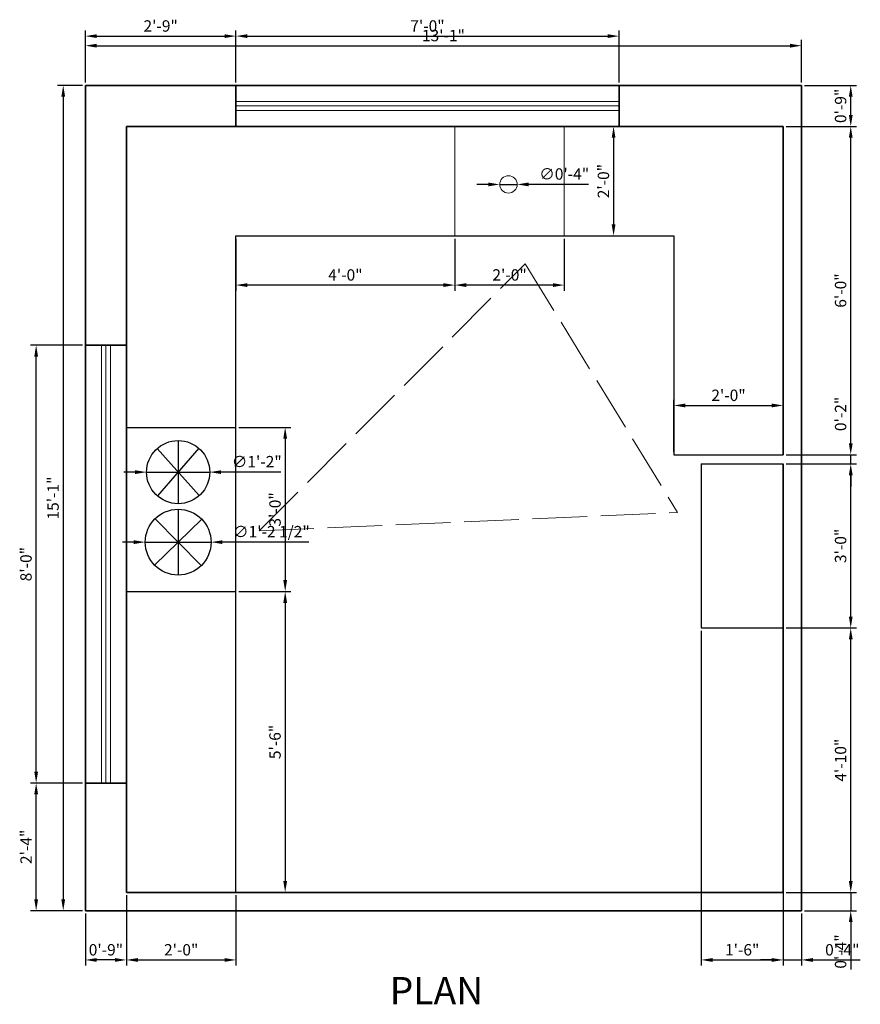
# Model space of a CAD drawing. Units: inches. Extents: x 125 to 951, y 142 to 358.
# Tile 1 of 4: x 125 to 309, y 142 to 358. Entities that reach past the tile are written whole.
import ezdxf

# ---------------------------------------------------------------- set-up
doc = ezdxf.new("R2010")
doc.units = ezdxf.units.IN
doc.linetypes.add('ACAD_ISO02W100', pattern=[15, 12, -3])
for name, color, linetype, lineweight in [('A-ANNO-DIMS', 2, 'Continuous', 18), ('A-ANNO-TEXT', 7, 'Continuous', 25), ('A-ANNO-WORK', 3, 'ACAD_ISO02W100', 13), ('A-EQPM', 8, 'Continuous', 25), ('A-FLOR-CNTR', 30, 'Continuous', 25), ('A-FLOR-FIXT', 9, 'Continuous', 18), ('A-GLAZ', 4, 'Continuous', 18), ('A-WALL', 7, 'Continuous', 35)]:
    doc.layers.add(name, color=color, linetype=linetype, lineweight=lineweight)
doc.styles.get("Standard").update_dxf_attribs({"font": 'arial.ttf'})
doc.dimstyles.new('ISO-25', dxfattribs={"dimtxt": 2.5, "dimasz": 2.5, "dimexe": 1.25, "dimexo": 0.625, "dimtad": 1, "dimlunit": 3, "dimtxsty": 'Standard', "dimcen": 2.5, "dimadec": 0, "dimazin": 0, "dimtfac": 1, "dimtmove": 0, "dimatfit": 3, "dimfxl": 1, "dimarcsym": 0})

# ---------------------------------------------------------------- blocks, each defined once
blk = doc.blocks.new('*D1')
at = {"layer": 'A-ANNO-DIMS', "color": 0, "lineweight": -2, "transparency": 16777216}
for p, q in [((138.96, 344.03), (138.96, 353.36)), ((141.46, 352.11), (293.46, 352.11)), ((295.96, 344.03), (295.96, 353.36))]:
    blk.add_line(p, q, dxfattribs=at)
at = {"layer": 'A-ANNO-DIMS', "color": 0, "transparency": 16777216}
for points in [[(141.46, 352.53), (141.46, 351.69), (138.96, 352.11)], [(293.46, 352.53), (293.46, 351.69), (295.96, 352.11)]]:
    blk.add_solid(points, dxfattribs=at)
at = {"layer": 'Defpoints', "color": 0, "transparency": 16777216}
for p in [(295.96, 352.11), (138.96, 343.41), (295.96, 343.41)]:
    blk.add_point(p, dxfattribs=at)
at = {"layer": 'A-ANNO-DIMS', "color": 0, "transparency": 16777216, "insert": (217.46, 354.01), "char_height": 2.5, "attachment_point": 5}
blk.add_mtext('13\'-1"', dxfattribs=at)
blk = doc.blocks.new('*D2')
at = {"layer": 'A-ANNO-DIMS', "color": 0, "lineweight": -2, "transparency": 16777216}
for p, q in [((138.34, 343.41), (132.85, 343.41)), ((134.1, 340.91), (134.1, 164.91)), ((138.34, 162.41), (132.85, 162.41))]:
    blk.add_line(p, q, dxfattribs=at)
at = {"layer": 'A-ANNO-DIMS', "color": 0, "transparency": 16777216}
for points in [[(133.68, 340.91), (134.51, 340.91), (134.1, 343.41)], [(133.68, 164.91), (134.51, 164.91), (134.1, 162.41)]]:
    blk.add_solid(points, dxfattribs=at)
at = {"layer": 'Defpoints', "color": 0, "transparency": 16777216}
for p in [(138.96, 343.41), (134.1, 162.41), (138.96, 162.41)]:
    blk.add_point(p, dxfattribs=at)
at = {"layer": 'A-ANNO-DIMS', "color": 0, "transparency": 16777216, "insert": (132.19, 252.91), "char_height": 2.5, "attachment_point": 5, "rotation": 90}
blk.add_mtext('15\'-1"', dxfattribs=at)
blk = doc.blocks.new('*D21')
at = {"layer": 'A-ANNO-DIMS', "color": 0, "lineweight": -2, "transparency": 16777216}
for p, q in [((138.96, 344.03), (138.96, 355.46)), ((141.46, 354.21), (169.46, 354.21)), ((171.96, 344.03), (171.96, 355.46))]:
    blk.add_line(p, q, dxfattribs=at)
at = {"layer": 'A-ANNO-DIMS', "color": 0, "transparency": 16777216}
for points in [[(141.46, 354.62), (141.46, 353.79), (138.96, 354.21)], [(169.46, 354.62), (169.46, 353.79), (171.96, 354.21)]]:
    blk.add_solid(points, dxfattribs=at)
at = {"layer": 'Defpoints', "color": 0, "transparency": 16777216}
for p in [(171.96, 354.21), (138.96, 343.41), (171.96, 343.41)]:
    blk.add_point(p, dxfattribs=at)
at = {"layer": 'A-ANNO-DIMS', "color": 0, "transparency": 16777216, "insert": (155.46, 356.11), "char_height": 2.5, "attachment_point": 5}
blk.add_mtext('2\'-9"', dxfattribs=at)
blk = doc.blocks.new('*D22')
at = {"layer": 'A-ANNO-DIMS', "color": 0, "lineweight": -2, "transparency": 16777216}
for p, q in [((171.96, 344.03), (171.96, 355.46)), ((174.46, 354.21), (253.46, 354.21)), ((255.96, 344.03), (255.96, 355.46))]:
    blk.add_line(p, q, dxfattribs=at)
at = {"layer": 'A-ANNO-DIMS', "color": 0, "transparency": 16777216}
for points in [[(174.46, 354.62), (174.46, 353.79), (171.96, 354.21)], [(253.46, 354.62), (253.46, 353.79), (255.96, 354.21)]]:
    blk.add_solid(points, dxfattribs=at)
at = {"layer": 'Defpoints', "color": 0, "transparency": 16777216}
for p in [(255.96, 354.21), (171.96, 343.41), (255.96, 343.41)]:
    blk.add_point(p, dxfattribs=at)
at = {"layer": 'A-ANNO-DIMS', "color": 0, "transparency": 16777216, "insert": (213.96, 356.11), "char_height": 2.5, "attachment_point": 5}
blk.add_mtext('7\'-0"', dxfattribs=at)
blk = doc.blocks.new('*D23')
at = {"layer": 'A-ANNO-DIMS', "color": 0, "lineweight": -2, "transparency": 16777216}
for p, q in [((138.34, 286.41), (126.91, 286.41)), ((128.16, 192.91), (128.16, 283.91)), ((138.34, 190.41), (126.91, 190.41))]:
    blk.add_line(p, q, dxfattribs=at)
at = {"layer": 'A-ANNO-DIMS', "color": 0, "transparency": 16777216}
for points in [[(127.75, 283.91), (128.58, 283.91), (128.16, 286.41)], [(127.75, 192.91), (128.58, 192.91), (128.16, 190.41)]]:
    blk.add_solid(points, dxfattribs=at)
at = {"layer": 'Defpoints', "color": 0, "transparency": 16777216}
for p in [(128.16, 286.41), (138.96, 286.41), (138.96, 190.41)]:
    blk.add_point(p, dxfattribs=at)
at = {"layer": 'A-ANNO-DIMS', "color": 0, "transparency": 16777216, "insert": (126.26, 238.41), "char_height": 2.5, "attachment_point": 5, "rotation": 90}
blk.add_mtext('8\'-0"', dxfattribs=at)
blk = doc.blocks.new('*D24')
at = {"layer": 'A-ANNO-DIMS', "color": 0, "lineweight": -2, "transparency": 16777216}
for p, q in [((138.34, 190.41), (126.91, 190.41)), ((128.16, 164.91), (128.16, 187.91)), ((138.34, 162.41), (126.91, 162.41))]:
    blk.add_line(p, q, dxfattribs=at)
at = {"layer": 'A-ANNO-DIMS', "color": 0, "transparency": 16777216}
for points in [[(127.75, 187.91), (128.58, 187.91), (128.16, 190.41)], [(127.75, 164.91), (128.58, 164.91), (128.16, 162.41)]]:
    blk.add_solid(points, dxfattribs=at)
at = {"layer": 'Defpoints', "color": 0, "transparency": 16777216}
for p in [(128.16, 190.41), (138.96, 190.41), (138.96, 162.41)]:
    blk.add_point(p, dxfattribs=at)
at = {"layer": 'A-ANNO-DIMS', "color": 0, "transparency": 16777216, "insert": (126.28, 176.41), "char_height": 2.5, "attachment_point": 5, "rotation": 90}
blk.add_mtext('2\'-4"', dxfattribs=at)
blk = doc.blocks.new('*D25')
at = {"layer": 'A-ANNO-DIMS', "color": 0, "lineweight": -2, "transparency": 16777216}
for p, q in [((147.96, 165.78), (147.96, 150.36)), ((171.96, 165.78), (171.96, 150.36)), ((150.46, 151.61), (169.46, 151.61))]:
    blk.add_line(p, q, dxfattribs=at)
at = {"layer": 'A-ANNO-DIMS', "color": 0, "transparency": 16777216}
for points in [[(150.46, 152.02), (150.46, 151.19), (147.96, 151.61)], [(169.46, 152.02), (169.46, 151.19), (171.96, 151.61)]]:
    blk.add_solid(points, dxfattribs=at)
at = {"layer": 'Defpoints', "color": 0, "transparency": 16777216}
for p in [(147.96, 166.41), (171.96, 166.41), (171.96, 151.61)]:
    blk.add_point(p, dxfattribs=at)
at = {"layer": 'A-ANNO-DIMS', "color": 0, "transparency": 16777216, "insert": (159.96, 153.51), "char_height": 2.5, "attachment_point": 5}
blk.add_mtext('2\'-0"', dxfattribs=at)
blk = doc.blocks.new('*D26')
at = {"layer": 'A-ANNO-DIMS', "color": 0, "lineweight": -2, "transparency": 16777216}
for p, q in [((171.96, 309.78), (171.96, 298.36)), ((219.96, 309.78), (219.96, 298.36)), ((217.46, 299.61), (174.46, 299.61))]:
    blk.add_line(p, q, dxfattribs=at)
at = {"layer": 'A-ANNO-DIMS', "color": 0, "transparency": 16777216}
for points in [[(174.46, 300.02), (174.46, 299.19), (171.96, 299.61)], [(217.46, 300.02), (217.46, 299.19), (219.96, 299.61)]]:
    blk.add_solid(points, dxfattribs=at)
at = {"layer": 'Defpoints', "color": 0, "transparency": 16777216}
for p in [(171.96, 310.41), (219.96, 310.41), (171.96, 299.61)]:
    blk.add_point(p, dxfattribs=at)
at = {"layer": 'A-ANNO-DIMS', "color": 0, "transparency": 16777216, "insert": (195.96, 301.51), "char_height": 2.5, "attachment_point": 5}
blk.add_mtext('4\'-0"', dxfattribs=at)
blk = doc.blocks.new('*D27')
at = {"layer": 'A-ANNO-DIMS', "color": 0, "lineweight": -2, "transparency": 16777216}
for p, q in [((219.96, 309.78), (219.96, 298.36)), ((243.96, 309.78), (243.96, 298.36)), ((241.46, 299.61), (222.46, 299.61))]:
    blk.add_line(p, q, dxfattribs=at)
at = {"layer": 'A-ANNO-DIMS', "color": 0, "transparency": 16777216}
for points in [[(222.46, 300.02), (222.46, 299.19), (219.96, 299.61)], [(241.46, 300.02), (241.46, 299.19), (243.96, 299.61)]]:
    blk.add_solid(points, dxfattribs=at)
at = {"layer": 'Defpoints', "color": 0, "transparency": 16777216}
for p in [(219.96, 310.41), (243.96, 310.41), (219.96, 299.61)]:
    blk.add_point(p, dxfattribs=at)
at = {"layer": 'A-ANNO-DIMS', "color": 0, "transparency": 16777216, "insert": (231.96, 301.51), "char_height": 2.5, "attachment_point": 5}
blk.add_mtext('2\'-0"', dxfattribs=at)
blk = doc.blocks.new('*D28')
at = {"layer": 'A-ANNO-DIMS', "color": 0, "lineweight": -2, "transparency": 16777216}
for p, q in [((172.59, 232.41), (184.01, 232.41)), ((182.76, 229.91), (182.76, 168.91)), ((172.59, 166.41), (184.01, 166.41))]:
    blk.add_line(p, q, dxfattribs=at)
at = {"layer": 'A-ANNO-DIMS', "color": 0, "transparency": 16777216}
for points in [[(182.35, 229.91), (183.18, 229.91), (182.76, 232.41)], [(182.35, 168.91), (183.18, 168.91), (182.76, 166.41)]]:
    blk.add_solid(points, dxfattribs=at)
at = {"layer": 'Defpoints', "color": 0, "transparency": 16777216}
for p in [(171.96, 232.41), (171.96, 166.41), (182.76, 166.41)]:
    blk.add_point(p, dxfattribs=at)
at = {"layer": 'A-ANNO-DIMS', "color": 0, "transparency": 16777216, "insert": (180.86, 199.41), "char_height": 2.5, "attachment_point": 5, "rotation": 90}
blk.add_mtext('5\'-6"', dxfattribs=at)
blk = doc.blocks.new('*D29')
at = {"layer": 'A-ANNO-DIMS', "color": 0, "lineweight": -2, "transparency": 16777216}
for p, q in [((172.59, 268.41), (184.01, 268.41)), ((182.76, 265.91), (182.76, 234.91)), ((172.59, 232.41), (184.01, 232.41))]:
    blk.add_line(p, q, dxfattribs=at)
at = {"layer": 'A-ANNO-DIMS', "color": 0, "transparency": 16777216}
for points in [[(182.35, 265.91), (183.18, 265.91), (182.76, 268.41)], [(182.35, 234.91), (183.18, 234.91), (182.76, 232.41)]]:
    blk.add_solid(points, dxfattribs=at)
at = {"layer": 'Defpoints', "color": 0, "transparency": 16777216}
for p in [(171.96, 268.41), (171.96, 232.41), (182.76, 232.41)]:
    blk.add_point(p, dxfattribs=at)
at = {"layer": 'A-ANNO-DIMS', "color": 0, "transparency": 16777216, "insert": (180.86, 250.41), "char_height": 2.5, "attachment_point": 5, "rotation": 90}
blk.add_mtext('3\'-0"', dxfattribs=at)
blk = doc.blocks.new('*D30')
at = {"layer": 'A-ANNO-DIMS', "color": 0, "lineweight": -2, "transparency": 16777216}
for p, q in [((292.59, 334.41), (308.01, 334.41)), ((306.76, 264.91), (306.76, 331.91)), ((292.59, 262.41), (308.01, 262.41))]:
    blk.add_line(p, q, dxfattribs=at)
at = {"layer": 'A-ANNO-DIMS', "color": 0, "transparency": 16777216}
for points in [[(306.35, 331.91), (307.18, 331.91), (306.76, 334.41)], [(306.35, 264.91), (307.18, 264.91), (306.76, 262.41)]]:
    blk.add_solid(points, dxfattribs=at)
at = {"layer": 'Defpoints', "color": 0, "transparency": 16777216}
for p in [(291.96, 334.41), (306.76, 334.41), (291.96, 262.41)]:
    blk.add_point(p, dxfattribs=at)
at = {"layer": 'A-ANNO-DIMS', "color": 0, "transparency": 16777216, "insert": (304.86, 298.41), "char_height": 2.5, "attachment_point": 5, "rotation": 90}
blk.add_mtext('6\'-0"', dxfattribs=at)
blk = doc.blocks.new('*D31')
at = {"layer": 'A-ANNO-DIMS', "color": 0, "lineweight": -2, "transparency": 16777216}
for p, q in [((273.96, 223.78), (273.96, 150.36)), ((291.96, 223.78), (291.96, 150.36)), ((276.46, 151.61), (289.46, 151.61))]:
    blk.add_line(p, q, dxfattribs=at)
at = {"layer": 'A-ANNO-DIMS', "color": 0, "transparency": 16777216}
for points in [[(276.46, 152.02), (276.46, 151.19), (273.96, 151.61)], [(289.46, 152.02), (289.46, 151.19), (291.96, 151.61)]]:
    blk.add_solid(points, dxfattribs=at)
at = {"layer": 'Defpoints', "color": 0, "transparency": 16777216}
for p in [(273.96, 224.41), (291.96, 224.41), (291.96, 151.61)]:
    blk.add_point(p, dxfattribs=at)
at = {"layer": 'A-ANNO-DIMS', "color": 0, "transparency": 16777216, "insert": (282.96, 153.51), "char_height": 2.5, "attachment_point": 5}
blk.add_mtext('1\'-6"', dxfattribs=at)
blk = doc.blocks.new('*D32')
at = {"layer": 'A-ANNO-DIMS', "color": 0, "lineweight": -2, "transparency": 16777216}
for p, q in [((292.59, 260.41), (308.01, 260.41)), ((306.76, 226.91), (306.76, 257.91)), ((292.59, 224.41), (308.01, 224.41))]:
    blk.add_line(p, q, dxfattribs=at)
at = {"layer": 'A-ANNO-DIMS', "color": 0, "transparency": 16777216}
for points in [[(306.35, 257.91), (307.18, 257.91), (306.76, 260.41)], [(306.35, 226.91), (307.18, 226.91), (306.76, 224.41)]]:
    blk.add_solid(points, dxfattribs=at)
at = {"layer": 'Defpoints', "color": 0, "transparency": 16777216}
for p in [(291.96, 260.41), (306.76, 260.41), (291.96, 224.41)]:
    blk.add_point(p, dxfattribs=at)
at = {"layer": 'A-ANNO-DIMS', "color": 0, "transparency": 16777216, "insert": (304.86, 242.41), "char_height": 2.5, "attachment_point": 5, "rotation": 90}
blk.add_mtext('3\'-0"', dxfattribs=at)
blk = doc.blocks.new('*D33')
at = {"layer": 'A-ANNO-DIMS', "color": 0, "lineweight": -2, "transparency": 16777216}
for p, q in [((292.59, 224.41), (308.01, 224.41)), ((306.76, 168.91), (306.76, 221.91)), ((292.59, 166.41), (308.01, 166.41))]:
    blk.add_line(p, q, dxfattribs=at)
at = {"layer": 'A-ANNO-DIMS', "color": 0, "transparency": 16777216}
for points in [[(306.35, 221.91), (307.18, 221.91), (306.76, 224.41)], [(306.35, 168.91), (307.18, 168.91), (306.76, 166.41)]]:
    blk.add_solid(points, dxfattribs=at)
at = {"layer": 'Defpoints', "color": 0, "transparency": 16777216}
for p in [(291.96, 224.41), (306.76, 224.41), (291.96, 166.41)]:
    blk.add_point(p, dxfattribs=at)
at = {"layer": 'A-ANNO-DIMS', "color": 0, "transparency": 16777216, "insert": (304.86, 195.41), "char_height": 2.5, "attachment_point": 5, "rotation": 90}
blk.add_mtext('4\'-10"', dxfattribs=at)
blk = doc.blocks.new('*D34')
at = {"layer": 'A-ANNO-DIMS', "color": 0, "lineweight": -2, "transparency": 16777216}
for p, q in [((147.96, 165.78), (147.96, 150.36)), ((138.96, 161.78), (138.96, 150.36)), ((145.46, 151.61), (141.46, 151.61))]:
    blk.add_line(p, q, dxfattribs=at)
at = {"layer": 'A-ANNO-DIMS', "color": 0, "transparency": 16777216}
for points in [[(141.46, 152.02), (141.46, 151.19), (138.96, 151.61)], [(145.46, 152.02), (145.46, 151.19), (147.96, 151.61)]]:
    blk.add_solid(points, dxfattribs=at)
at = {"layer": 'Defpoints', "color": 0, "transparency": 16777216}
for p in [(147.96, 166.41), (138.96, 162.41), (138.96, 151.61)]:
    blk.add_point(p, dxfattribs=at)
at = {"layer": 'A-ANNO-DIMS', "color": 0, "transparency": 16777216, "insert": (143.46, 153.51), "char_height": 2.5, "attachment_point": 5}
blk.add_mtext('0\'-9"', dxfattribs=at)
blk = doc.blocks.new('*D35')
at = {"layer": 'A-ANNO-DIMS', "color": 0, "lineweight": -2, "transparency": 16777216}
for p, q in [((291.96, 165.78), (291.96, 150.36)), ((295.96, 161.78), (295.96, 150.36)), ((289.46, 151.61), (286.96, 151.61)), ((291.96, 151.61), (295.96, 151.61)), ((298.46, 151.61), (308.86, 151.61))]:
    blk.add_line(p, q, dxfattribs=at)
at = {"layer": 'A-ANNO-DIMS', "color": 0, "transparency": 16777216}
for points in [[(289.46, 152.02), (289.46, 151.19), (291.96, 151.61)], [(298.46, 152.02), (298.46, 151.19), (295.96, 151.61)]]:
    blk.add_solid(points, dxfattribs=at)
at = {"layer": 'Defpoints', "color": 0, "transparency": 16777216}
for p in [(291.96, 166.41), (295.96, 162.41), (295.96, 151.61)]:
    blk.add_point(p, dxfattribs=at)
at = {"layer": 'A-ANNO-DIMS', "color": 0, "transparency": 16777216, "insert": (304.91, 153.51), "char_height": 2.5, "attachment_point": 5}
blk.add_mtext('0\'-4"', dxfattribs=at)
blk = doc.blocks.new('*D36')
at = {"layer": 'A-ANNO-DIMS', "color": 0, "lineweight": -2, "transparency": 16777216}
for p, q in [((296.59, 343.41), (308.01, 343.41)), ((306.76, 336.91), (306.76, 340.91)), ((292.59, 334.41), (308.01, 334.41))]:
    blk.add_line(p, q, dxfattribs=at)
at = {"layer": 'A-ANNO-DIMS', "color": 0, "transparency": 16777216}
for points in [[(306.35, 340.91), (307.18, 340.91), (306.76, 343.41)], [(306.35, 336.91), (307.18, 336.91), (306.76, 334.41)]]:
    blk.add_solid(points, dxfattribs=at)
at = {"layer": 'Defpoints', "color": 0, "transparency": 16777216}
for p in [(295.96, 343.41), (306.76, 343.41), (291.96, 334.41)]:
    blk.add_point(p, dxfattribs=at)
at = {"layer": 'A-ANNO-DIMS', "color": 0, "transparency": 16777216, "insert": (304.86, 338.91), "char_height": 2.5, "attachment_point": 5, "rotation": 90}
blk.add_mtext('0\'-9"', dxfattribs=at)
blk = doc.blocks.new('*D37')
at = {"layer": 'A-ANNO-DIMS', "color": 0, "lineweight": -2, "transparency": 16777216}
for p, q in [((306.76, 168.91), (306.76, 171.41)), ((292.59, 166.41), (308.01, 166.41)), ((306.76, 166.41), (306.76, 162.41)), ((296.59, 162.41), (308.01, 162.41)), ((306.76, 159.91), (306.76, 149.51))]:
    blk.add_line(p, q, dxfattribs=at)
at = {"layer": 'A-ANNO-DIMS', "color": 0, "transparency": 16777216}
for points in [[(306.35, 168.91), (307.18, 168.91), (306.76, 166.41)], [(306.35, 159.91), (307.18, 159.91), (306.76, 162.41)]]:
    blk.add_solid(points, dxfattribs=at)
at = {"layer": 'Defpoints', "color": 0, "transparency": 16777216}
for p in [(291.96, 166.41), (295.96, 162.41), (306.76, 162.41)]:
    blk.add_point(p, dxfattribs=at)
at = {"layer": 'A-ANNO-DIMS', "color": 0, "transparency": 16777216, "insert": (304.86, 153.46), "char_height": 2.5, "attachment_point": 5, "rotation": 90}
blk.add_mtext('0\'-4"', dxfattribs=at)
blk = doc.blocks.new('*D38')
at = {"layer": 'A-ANNO-DIMS', "color": 0, "lineweight": -2, "transparency": 16777216}
for p, q in [((244.59, 334.41), (256.01, 334.41)), ((254.76, 331.91), (254.76, 312.91)), ((244.59, 310.41), (256.01, 310.41))]:
    blk.add_line(p, q, dxfattribs=at)
at = {"layer": 'A-ANNO-DIMS', "color": 0, "transparency": 16777216}
for points in [[(254.35, 331.91), (255.18, 331.91), (254.76, 334.41)], [(254.35, 312.91), (255.18, 312.91), (254.76, 310.41)]]:
    blk.add_solid(points, dxfattribs=at)
at = {"layer": 'Defpoints', "color": 0, "transparency": 16777216}
for p in [(243.96, 334.41), (243.96, 310.41), (254.76, 310.41)]:
    blk.add_point(p, dxfattribs=at)
at = {"layer": 'A-ANNO-DIMS', "color": 0, "transparency": 16777216, "insert": (252.86, 322.41), "char_height": 2.5, "attachment_point": 5, "rotation": 90}
blk.add_mtext('2\'-0"', dxfattribs=at)
blk = doc.blocks.new('*D39')
at = {"layer": 'A-ANNO-DIMS', "color": 0, "lineweight": -2, "transparency": 16777216}
for p, q in [((267.96, 263.03), (267.96, 274.46)), ((291.96, 263.03), (291.96, 274.46)), ((270.46, 273.21), (289.46, 273.21))]:
    blk.add_line(p, q, dxfattribs=at)
at = {"layer": 'A-ANNO-DIMS', "color": 0, "transparency": 16777216}
for points in [[(270.46, 273.62), (270.46, 272.79), (267.96, 273.21)], [(289.46, 273.62), (289.46, 272.79), (291.96, 273.21)]]:
    blk.add_solid(points, dxfattribs=at)
at = {"layer": 'Defpoints', "color": 0, "transparency": 16777216}
for p in [(291.96, 273.21), (267.96, 262.41), (291.96, 262.41)]:
    blk.add_point(p, dxfattribs=at)
at = {"layer": 'A-ANNO-DIMS', "color": 0, "transparency": 16777216, "insert": (279.96, 275.11), "char_height": 2.5, "attachment_point": 5}
blk.add_mtext('2\'-0"', dxfattribs=at)
blk = doc.blocks.new('*D40')
at = {"layer": 'A-ANNO-DIMS', "color": 0, "lineweight": -2, "transparency": 16777216}
for p, q in [((306.76, 264.91), (306.76, 275.3)), ((292.59, 262.41), (308.01, 262.41)), ((306.76, 260.41), (306.76, 262.41)), ((292.59, 260.41), (308.01, 260.41)), ((306.76, 257.91), (306.76, 255.41))]:
    blk.add_line(p, q, dxfattribs=at)
at = {"layer": 'A-ANNO-DIMS', "color": 0, "transparency": 16777216}
for points in [[(306.35, 264.91), (307.18, 264.91), (306.76, 262.41)], [(306.35, 257.91), (307.18, 257.91), (306.76, 260.41)]]:
    blk.add_solid(points, dxfattribs=at)
at = {"layer": 'Defpoints', "color": 0, "transparency": 16777216}
for p in [(291.96, 262.41), (306.76, 262.41), (291.96, 260.41)]:
    blk.add_point(p, dxfattribs=at)
at = {"layer": 'A-ANNO-DIMS', "color": 0, "transparency": 16777216, "insert": (304.86, 271.35), "char_height": 2.5, "attachment_point": 5, "rotation": 90}
blk.add_mtext('0\'-2"', dxfattribs=at)
blk = doc.blocks.new('*D72')
at = {"layer": 'A-ANNO-DIMS', "color": 0, "lineweight": -2, "transparency": 16777216}
for p, q in [((149.57, 243.23), (147.07, 243.23)), ((152.07, 243.23), (166.52, 243.23)), ((187.96, 243.23), (169.02, 243.23))]:
    blk.add_line(p, q, dxfattribs=at)
at = {"layer": 'A-ANNO-DIMS', "color": 0, "transparency": 16777216}
for points in [[(149.57, 243.65), (149.57, 242.82), (152.07, 243.23)], [(169.02, 243.65), (169.02, 242.82), (166.52, 243.23)]]:
    blk.add_solid(points, dxfattribs=at)
at = {"layer": 'Defpoints', "color": 0, "transparency": 16777216}
for p in [(152.07, 243.23), (166.52, 243.23)]:
    blk.add_point(p, dxfattribs=at)
at = {"layer": 'A-ANNO-DIMS', "color": 0, "transparency": 16777216, "insert": (179.74, 245.21), "char_height": 2.5, "attachment_point": 5, "rotation": 0.0037}
blk.add_mtext('∅1\'-2 1/2"', dxfattribs=at)
blk = doc.blocks.new('*D73')
at = {"layer": 'A-ANNO-DIMS', "color": 0, "lineweight": -2, "transparency": 16777216}
for p, q in [((149.87, 258.59), (147.37, 258.59)), ((152.37, 258.59), (166.22, 258.59)), ((181.84, 258.59), (168.72, 258.59))]:
    blk.add_line(p, q, dxfattribs=at)
at = {"layer": 'A-ANNO-DIMS', "color": 0, "transparency": 16777216}
for points in [[(149.87, 259), (149.87, 258.17), (152.37, 258.59)], [(168.72, 259), (168.72, 258.17), (166.22, 258.59)]]:
    blk.add_solid(points, dxfattribs=at)
at = {"layer": 'Defpoints', "color": 0, "transparency": 16777216}
for p in [(152.37, 258.59), (166.22, 258.59)]:
    blk.add_point(p, dxfattribs=at)
at = {"layer": 'A-ANNO-DIMS', "color": 0, "transparency": 16777216, "insert": (176.53, 260.56), "char_height": 2.5, "attachment_point": 5, "rotation": 359.9994}
blk.add_mtext('∅1\'-2"', dxfattribs=at)
blk = doc.blocks.new('*D74')
at = {"layer": 'A-ANNO-DIMS', "color": 0, "lineweight": -2, "transparency": 16777216}
for p, q in [((227.3, 321.68), (224.8, 321.68)), ((229.8, 321.68), (233.63, 321.68)), ((249.24, 321.68), (236.13, 321.68))]:
    blk.add_line(p, q, dxfattribs=at)
at = {"layer": 'A-ANNO-DIMS', "color": 0, "transparency": 16777216}
for points in [[(227.3, 322.1), (227.3, 321.27), (229.8, 321.68)], [(236.13, 322.1), (236.13, 321.27), (233.63, 321.68)]]:
    blk.add_solid(points, dxfattribs=at)
at = {"layer": 'Defpoints', "color": 0, "transparency": 16777216}
for p in [(229.8, 321.68), (233.63, 321.68)]:
    blk.add_point(p, dxfattribs=at)
at = {"layer": 'A-ANNO-DIMS', "color": 0, "transparency": 16777216, "insert": (243.94, 323.65), "char_height": 2.5, "attachment_point": 5, "rotation": 0.0018}
blk.add_mtext('∅0\'-4"', dxfattribs=at)

msp = doc.modelspace()

# ---------------------------------------------------------------- linework, layer by layer
at = {"layer": 'A-ANNO-WORK'}
for p, q in [((177.071, 245.7), (235.414, 304.284)), ((235.414, 304.284), (268.795, 249.76)), ((177.071, 245.7), (268.795, 249.76))]:
    msp.add_line(p, q, dxfattribs=at)
at = {"layer": 'A-EQPM'}
for p, q in [((147.962, 268.406), (171.962, 268.406)), ((154.679, 263.744), (163.917, 253.428)), ((163.836, 263.816), (154.76, 253.356)), ((159.298, 265.51), (159.298, 251.662)), ((273.962, 260.406), (291.962, 260.406)), ((273.962, 260.406), (273.962, 224.406)), ((152.374, 258.586), (166.222, 258.586)), ((154.228, 248.38), (164.369, 238.086)), ((159.298, 250.458), (159.298, 236.007)), ((164.466, 248.282), (154.13, 238.183)), ((152.073, 243.233), (166.523, 243.233)), ((147.962, 232.406), (171.962, 232.406)), ((273.962, 224.406), (291.962, 224.406))]:
    msp.add_line(p, q, dxfattribs=at)
for centre, radius in [((159.298, 258.586), 6.924), ((159.298, 243.233), 7.225)]:
    msp.add_circle(centre, radius, dxfattribs=at)
at = {"layer": 'A-FLOR-CNTR'}
for p, q in [((171.962, 310.406), (267.962, 310.406)), ((171.962, 166.406), (171.962, 310.406)), ((267.962, 310.406), (267.962, 262.406)), ((267.962, 262.406), (291.962, 262.406))]:
    msp.add_line(p, q, dxfattribs=at)
at = {"layer": 'A-FLOR-FIXT'}
for p, q in [((219.962, 310.406), (219.962, 334.406)), ((243.962, 310.406), (243.962, 334.406))]:
    msp.add_line(p, q, dxfattribs=at)
msp.add_circle((231.716, 321.683), 1.912, dxfattribs=at)
at = {"layer": 'A-GLAZ'}
for p, q in [((171.962, 339.906), (255.962, 339.906)), ((171.962, 338.906), (255.962, 338.906)), ((171.962, 337.906), (255.962, 337.906)), ((142.462, 286.406), (142.462, 190.406)), ((143.462, 286.406), (143.462, 190.406)), ((144.462, 286.406), (144.462, 190.406))]:
    msp.add_line(p, q, dxfattribs=at)
at = {"layer": 'A-WALL'}
for p, q in [((138.962, 334.406), (138.962, 343.406)), ((138.962, 343.406), (147.962, 343.406)), ((147.962, 343.406), (291.962, 343.406)), ((171.962, 334.406), (171.962, 343.406)), ((255.962, 334.406), (255.962, 343.406)), ((291.962, 343.406), (295.962, 343.406)), ((295.962, 343.406), (295.962, 334.406)), ((138.962, 166.406), (138.962, 334.406)), ((147.962, 334.406), (291.962, 334.406)), ((147.962, 166.406), (147.962, 334.406)), ((147.962, 334.406), (171.962, 334.406)), ((291.962, 334.406), (291.962, 262.406)), ((295.962, 334.406), (295.962, 166.406)), ((147.962, 286.406), (138.962, 286.406)), ((291.962, 260.406), (291.962, 166.406)), ((147.962, 190.406), (138.962, 190.406)), ((147.962, 166.406), (147.962, 190.406)), ((138.962, 166.406), (138.962, 162.406)), ((291.962, 166.406), (147.962, 166.406)), ((295.962, 166.406), (295.962, 162.406)), ((291.962, 162.406), (138.962, 162.406)), ((295.962, 162.406), (291.962, 162.406))]:
    msp.add_line(p, q, dxfattribs=at)

# ---------------------------------------------------------------- texts
at = {"layer": 'A-ANNO-TEXT', "insert": (205.663, 147.879), "char_height": 6, "attachment_point": 1}
msp.add_mtext_dynamic_manual_height_columns('PLAN', width=92.57299, gutter_width=12.5, heights=[0], dxfattribs=at)

# ---------------------------------------------------------------- dimensions: what is measured, and where the dimension line sits
at = {"layer": 'A-ANNO-DIMS'}
for base, p1, p2, override, picture, middle in [((171.962, 354.206), (138.962, 343.406), (171.962, 343.406), {"dimdec": 1, "dimlfac": 1, "dimrnd": 0, "dimzin": 1, "dimdsep": 46, "dimlunit": 4, "dimfrac": 2}, '*D21', (155.462, 356.107)), ((255.962, 354.206), (171.962, 343.406), (255.962, 343.406), {"dimdec": 1, "dimlfac": 1, "dimrnd": 0, "dimzin": 1, "dimdsep": 46, "dimlunit": 4, "dimfrac": 2}, '*D22', (213.962, 356.107)), ((295.962, 352.111), (138.962, 343.406), (295.962, 343.406), {"dimclrd": 0, "dimclre": 0, "dimclrt": 0}, '*D1', (217.462, 354.013)), ((291.962, 273.206), (267.962, 262.406), (291.962, 262.406), {"dimdec": 1, "dimlfac": 1, "dimrnd": 0, "dimzin": 1, "dimdsep": 46, "dimlunit": 4, "dimfrac": 2}, '*D39', (279.962, 275.107)), ((291.962, 151.606), (273.962, 224.406), (291.962, 224.406), {"dimdec": 1, "dimlfac": 1, "dimrnd": 0, "dimzin": 1, "dimdsep": 46, "dimlunit": 4, "dimfrac": 2}, '*D31', (282.962, 153.507)), ((138.962, 151.606), (147.962, 166.406), (138.962, 162.406), {"dimdec": 1, "dimlfac": 1, "dimrnd": 0, "dimzin": 1, "dimdsep": 46, "dimlunit": 4, "dimfrac": 2}, '*D34', (143.462, 153.507)), ((171.962, 151.606), (147.962, 166.406), (171.962, 166.406), {"dimdec": 1, "dimlfac": 1, "dimrnd": 0, "dimzin": 1, "dimdsep": 46, "dimlunit": 4, "dimfrac": 2}, '*D25', (159.962, 153.507)), ((295.962, 151.606), (291.962, 166.406), (295.962, 162.406), {"dimdec": 1, "dimlfac": 1, "dimrnd": 0, "dimzin": 1, "dimdsep": 46, "dimlunit": 4, "dimfrac": 2}, '*D35', (304.909, 153.507))]:
    dim = msp.add_linear_dim(base=base, p1=p1, p2=p2, dimstyle='ISO-25', override=override, dxfattribs=at)
    dim.commit()
    dim.dimension.update_dxf_attribs({"geometry": picture, "text_midpoint": middle})
for base, p1, p2, angle, override, picture, middle in [((134.095, 162.406), (138.962, 343.406), (138.962, 162.406), 90, {"dimclrd": 0, "dimclre": 0, "dimclrt": 0}, '*D2', (132.194, 252.906)), ((306.762, 343.406), (291.962, 334.406), (295.962, 343.406), 90, {"dimdec": 1, "dimlfac": 1, "dimrnd": 0, "dimzin": 1, "dimdsep": 46, "dimlunit": 4, "dimfrac": 2}, '*D36', (304.86, 338.906)), ((254.762, 310.406), (243.962, 334.406), (243.962, 310.406), 270, {"dimdec": 1, "dimlfac": 1, "dimrnd": 0, "dimzin": 1, "dimdsep": 46, "dimlunit": 4, "dimfrac": 2}, '*D38', (252.86, 322.406)), ((306.762, 334.406), (291.962, 262.406), (291.962, 334.406), 90, {"dimdec": 1, "dimlfac": 1, "dimrnd": 0, "dimzin": 1, "dimdsep": 46, "dimlunit": 4, "dimfrac": 2}, '*D30', (304.86, 298.406)), ((171.962, 299.606), (219.962, 310.406), (171.962, 310.406), 180, {"dimdec": 1, "dimlfac": 1, "dimrnd": 0, "dimzin": 1, "dimdsep": 46, "dimlunit": 4, "dimfrac": 2}, '*D26', (195.962, 301.507)), ((219.962, 299.606), (243.962, 310.406), (219.962, 310.406), 180, {"dimdec": 1, "dimlfac": 1, "dimrnd": 0, "dimzin": 1, "dimdsep": 46, "dimlunit": 4, "dimfrac": 2}, '*D27', (231.962, 301.507)), ((128.162, 286.406), (138.962, 190.406), (138.962, 286.406), 90, {"dimdec": 1, "dimlfac": 1, "dimrnd": 0, "dimzin": 1, "dimdsep": 46, "dimlunit": 4, "dimfrac": 2}, '*D23', (126.26, 238.406)), ((306.762, 262.406), (291.962, 260.406), (291.962, 262.406), 90, {"dimdec": 1, "dimlfac": 1, "dimrnd": 0, "dimzin": 1, "dimdsep": 46, "dimlunit": 4, "dimfrac": 2}, '*D40', (304.86, 271.354)), ((182.762, 232.406), (171.962, 268.406), (171.962, 232.406), 270, {"dimdec": 1, "dimlfac": 1, "dimrnd": 0, "dimzin": 1, "dimdsep": 46, "dimlunit": 4, "dimfrac": 2}, '*D29', (180.859, 250.406)), ((306.762, 260.406), (291.962, 224.406), (291.962, 260.406), 90, {"dimdec": 1, "dimlfac": 1, "dimrnd": 0, "dimzin": 1, "dimdsep": 46, "dimlunit": 4, "dimfrac": 2}, '*D32', (304.859, 242.406)), ((182.762, 166.406), (171.962, 232.406), (171.962, 166.406), 270, {"dimdec": 1, "dimlfac": 1, "dimrnd": 0, "dimzin": 1, "dimdsep": 46, "dimlunit": 4, "dimfrac": 2}, '*D28', (180.86, 199.406)), ((306.762, 224.406), (291.962, 166.406), (291.962, 224.406), 90, {"dimdec": 1, "dimlfac": 1, "dimrnd": 0, "dimzin": 1, "dimdsep": 46, "dimlunit": 4, "dimfrac": 2}, '*D33', (304.86, 195.406)), ((128.162, 190.406), (138.962, 162.406), (138.962, 190.406), 90, {"dimdec": 1, "dimlfac": 1, "dimrnd": 0, "dimzin": 1, "dimdsep": 46, "dimlunit": 4, "dimfrac": 2}, '*D24', (126.282, 176.406)), ((306.762, 162.406), (291.962, 166.406), (295.962, 162.406), 90, {"dimdec": 1, "dimlfac": 1, "dimrnd": 0, "dimzin": 1, "dimdsep": 46, "dimlunit": 4, "dimfrac": 2}, '*D37', (304.86, 153.458))]:
    dim = msp.add_linear_dim(base=base, p1=p1, p2=p2, angle=angle, dimstyle='ISO-25', override=override, dxfattribs=at)
    dim.commit()
    dim.dimension.update_dxf_attribs({"geometry": picture, "text_midpoint": middle})
dim = msp.add_diameter_dim_2p(p1=(229.804, 321.683), p2=(233.628, 321.683), dimstyle='ISO-25', override={"dimdec": 1, "dimlfac": 1, "dimrnd": 0, "dimzin": 1, "dimdsep": 46, "dimlunit": 4, "dimfrac": 2}, dxfattribs=at)
dim.commit()
dim.dimension.update_dxf_attribs({"geometry": '*D74', "text_midpoint": (243.936, 321.683)})
for p1, p2, picture, middle in [((152.374, 258.586), (166.222, 258.586), '*D73', (176.53, 258.586)), ((152.073, 243.232), (166.523, 243.233), '*D72', (179.744, 243.234))]:
    dim = msp.add_diameter_dim_2p(p1=p1, p2=p2, dimstyle='ISO-25', override={"dimdec": 1, "dimlfac": 1, "dimrnd": 0, "dimzin": 1, "dimdsep": 46, "dimlunit": 4, "dimfrac": 2}, dxfattribs=at)
    dim.commit()
    dim.dimension.update_dxf_attribs({"geometry": picture, "text_midpoint": middle, "dimtype": 163})

doc.saveas('drawing.dxf')
